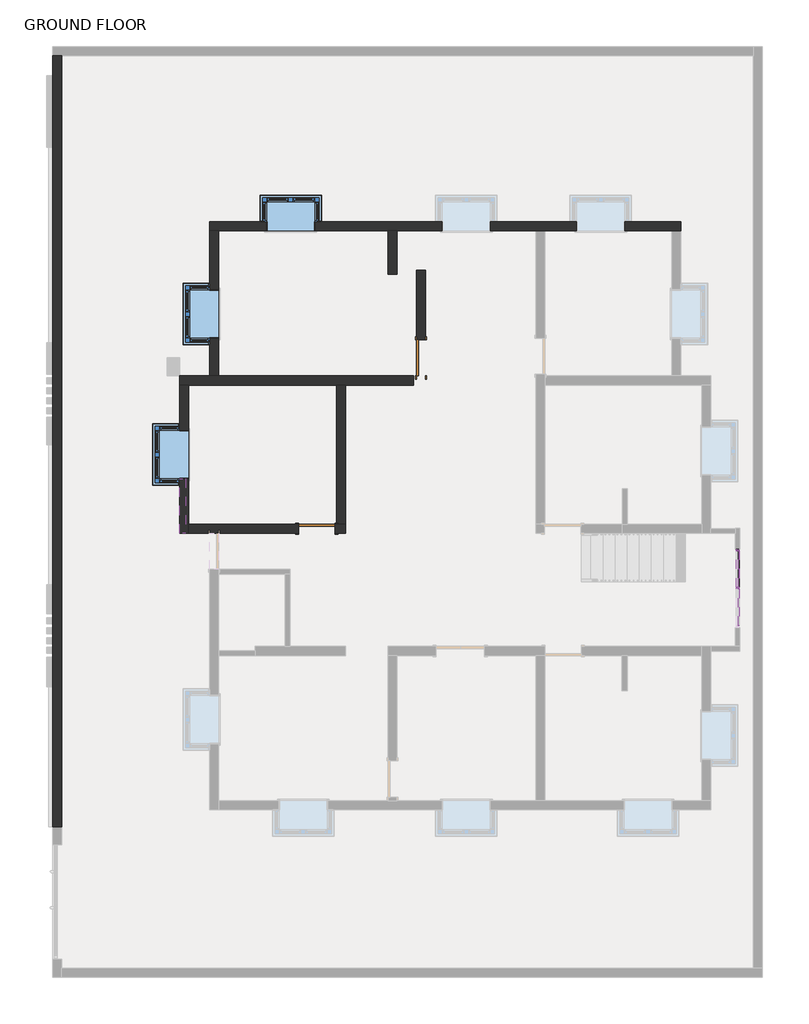
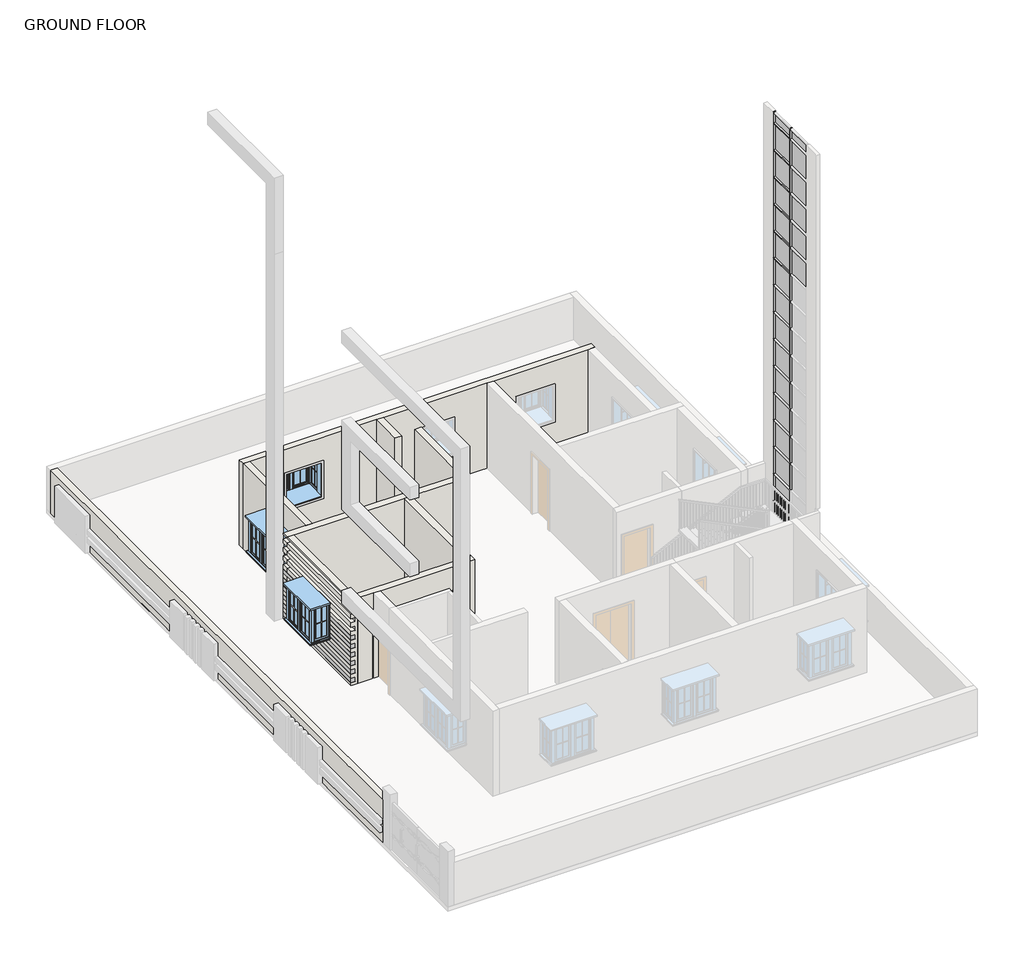
# One storey, part 2 of 5: 38 members, 23 plates, 9 walls, 6 proxies, 3 windows, 2 doors.
"""IFC4 building model written with IfcOpenShell, lengths in millimetres."""

from ifc_helpers import new_model, si_unit, frame, origin, origin_with_axes, place, context, project, spatial, polyline, outline, extrude, faceted_brep, transform, mapped, element, save
from components import door_a90ba1ad, door_0ca8825f, member_c65a811d, member_51048147, member_1ede677d, member_eea045b6, member_18929904, member_e7145701, member_32999801, system_panel_glazed_7f04015b, system_panel_glazed_95b6fecb, window_bay_casement_box_90_degree_angle_4_x4_x2_07b705a1

model = new_model("IFC4")

# Units and contexts
model_context = context("Model", 3, world=origin())
ifc_project = project(units=[si_unit("LENGTHUNIT", "METRE", prefix="MILLI")], contexts=[model_context])

# Site, building, storey
site = spatial("IfcSite", under=ifc_project)
building = spatial("IfcBuilding", under=site)
storey = spatial("IfcBuildingStorey", under=building, Name="GROUND FLOOR", Elevation=0.0)

# Proxies
placement = place(None, origin())
element("IfcBuildingElementProxy", 1, Name="Reveal", ObjectType="Reveal", at=placement, inside=storey, context=model_context, shape_type="SweptSolid", body=[
    extrude(outline(polyline([(-7008.3415084, 4183.133346), (-6855.9415084, 4183.133346), (-6855.9415084, 220.733346), (-7008.3415084, 220.733346), (-7008.3415084, 4183.133346)])), frame((0.0, 0.0, 101.6), z_axis=(0.0, 0.0, 1.0), x_axis=(1.0, 0.0, 0.0)), (0.0, 0.0, 1.0), 152.4),
])
element("IfcBuildingElementProxy", 2, Name="Reveal", ObjectType="Reveal", at=placement, inside=storey, context=model_context, shape_type="SweptSolid", body=[
    extrude(outline(polyline([(-7008.3415084, 4183.133346), (-6855.9415084, 4183.133346), (-6855.9415084, 220.733346), (-7008.3415084, 220.733346), (-7008.3415084, 4183.133346)])), frame((0.0, 0.0, 406.4), z_axis=(0.0, 0.0, 1.0), x_axis=(1.0, 0.0, 0.0)), (0.0, 0.0, 1.0), 152.4),
])
element("IfcBuildingElementProxy", 3, Name="Reveal", ObjectType="Reveal", at=placement, inside=storey, context=model_context, shape_type="SweptSolid", body=[
    extrude(outline(polyline([(-7008.3415084, 4183.133346), (-6855.9415084, 4183.133346), (-6855.9415084, 220.733346), (-7008.3415084, 220.733346), (-7008.3415084, 4183.133346)])), frame((0.0, 0.0, 711.2), z_axis=(0.0, 0.0, 1.0), x_axis=(1.0, 0.0, 0.0)), (0.0, 0.0, 1.0), 152.4),
])
element("IfcBuildingElementProxy", 4, Name="Reveal", ObjectType="Reveal", at=placement, inside=storey, context=model_context, shape_type="SweptSolid", body=[
    extrude(outline(polyline([(-7008.3415084, 1592.333346), (-6855.9415084, 1592.333346), (-6855.9415084, 220.733346), (-7008.3415084, 220.733346), (-7008.3415084, 1592.333346)])), frame((0.0, 0.0, 1016.0), z_axis=(0.0, 0.0, 1.0), x_axis=(1.0, 0.0, 0.0)), (0.0, 0.0, 1.0), 152.4),
    extrude(outline(polyline([(-7008.3415084, 4183.133346), (-6855.9415084, 4183.133346), (-6855.9415084, 2811.533346), (-7008.3415084, 2811.533346), (-7008.3415084, 4183.133346)])), frame((0.0, 0.0, 1016.0), z_axis=(0.0, 0.0, 1.0), x_axis=(1.0, 0.0, 0.0)), (0.0, 0.0, 1.0), 152.4),
])
element("IfcBuildingElementProxy", 5, Name="Reveal", ObjectType="Reveal", at=placement, inside=storey, context=model_context, shape_type="SweptSolid", body=[
    extrude(outline(polyline([(-7008.3415084, 1592.333346), (-6855.9415084, 1592.333346), (-6855.9415084, 220.733346), (-7008.3415084, 220.733346), (-7008.3415084, 1592.333346)])), frame((0.0, 0.0, 1320.8), z_axis=(0.0, 0.0, 1.0), x_axis=(1.0, 0.0, 0.0)), (0.0, 0.0, 1.0), 152.4),
    extrude(outline(polyline([(-7008.3415084, 4183.133346), (-6855.9415084, 4183.133346), (-6855.9415084, 2811.533346), (-7008.3415084, 2811.533346), (-7008.3415084, 4183.133346)])), frame((0.0, 0.0, 1320.8), z_axis=(0.0, 0.0, 1.0), x_axis=(1.0, 0.0, 0.0)), (0.0, 0.0, 1.0), 152.4),
])
element("IfcBuildingElementProxy", 6, Name="Reveal", ObjectType="Reveal", at=placement, inside=storey, context=model_context, shape_type="SweptSolid", body=[
    extrude(outline(polyline([(-7008.3415084, 1592.333346), (-6855.9415084, 1592.333346), (-6855.9415084, 220.733346), (-7008.3415084, 220.733346), (-7008.3415084, 1592.333346)])), frame((0.0, 0.0, 1625.6), z_axis=(0.0, 0.0, 1.0), x_axis=(1.0, 0.0, 0.0)), (0.0, 0.0, 1.0), 152.4),
    extrude(outline(polyline([(-7008.3415084, 4183.133346), (-6855.9415084, 4183.133346), (-6855.9415084, 2811.533346), (-7008.3415084, 2811.533346), (-7008.3415084, 4183.133346)])), frame((0.0, 0.0, 1625.6), z_axis=(0.0, 0.0, 1.0), x_axis=(1.0, 0.0, 0.0)), (0.0, 0.0, 1.0), 152.4),
])

# Doors
door_shape = door_a90ba1ad(model_context)
element("IfcDoor", 7, ObjectType="Single-Flush : 36\" x 84\"", at=placement, inside=storey, context=model_context, shape_type="MappedRepresentation", body=[
    mapped(door_shape, transform((-918.5024437, 4640.333346, 0.0), x_axis=(0.0, -1.0, 0.0), y_axis=(1.0, 0.0, 0.0), z_axis=(0.0, 0.0, 1.0))),
])
door_2_shape = door_0ca8825f(model_context)
element("IfcDoor", 8, ObjectType="Single-Flush : 36\" x 84\"", at=placement, inside=storey, context=model_context, shape_type="MappedRepresentation", body=[
    mapped(door_2_shape, transform((-3541.2415084, 335.033346, 0.0), x_axis=(1.0, 0.0, 0.0), y_axis=(0.0, 1.0, 0.0), z_axis=(0.0, 0.0, 1.0))),
])

# Members
member_shape = member_c65a811d(model_context)
element("IfcMember", 9, ObjectType="Rectangular Mullion : 1.5\" x 2.5\" rectangular", at=placement, inside=storey, context=model_context, shape_type="MappedRepresentation", body=[
    mapped(member_shape, transform((7067.5550459, -219.956654, 0.0), x_axis=(0.0, 0.0, -1.0), y_axis=(-1.0, 0.0, 0.0), z_axis=(0.0, 1.0, 0.0))),
])
member_2_shape = member_51048147(model_context)
element("IfcMember", 10, ObjectType="Rectangular Mullion : 1.5\" x 2.5\" rectangular", at=placement, inside=storey, context=model_context, shape_type="MappedRepresentation", body=[
    mapped(member_2_shape, transform((7067.5550459, -1147.0566543, 10636.25), x_axis=(0.0, 0.0, 1.0), y_axis=(-1.0, 0.0, 0.0), z_axis=(0.0, -1.0, 0.0))),
])
element("IfcMember", 11, ObjectType="Rectangular Mullion : 1.5\" x 2.5\" rectangular", at=placement, inside=storey, context=model_context, shape_type="MappedRepresentation", body=[
    mapped(member_2_shape, transform((7067.5550459, -1147.0566543, 11601.45), x_axis=(0.0, 0.0, 1.0), y_axis=(-1.0, 0.0, 0.0), z_axis=(0.0, -1.0, 0.0))),
])
element("IfcMember", 12, ObjectType="Rectangular Mullion : 1.5\" x 2.5\" rectangular", at=placement, inside=storey, context=model_context, shape_type="MappedRepresentation", body=[
    mapped(member_2_shape, transform((7067.5550459, -1147.0566543, 12566.65), x_axis=(0.0, 0.0, 1.0), y_axis=(-1.0, 0.0, 0.0), z_axis=(0.0, -1.0, 0.0))),
])
element("IfcMember", 13, ObjectType="Rectangular Mullion : 1.5\" x 2.5\" rectangular", at=placement, inside=storey, context=model_context, shape_type="MappedRepresentation", body=[
    mapped(member_2_shape, transform((7067.5550459, -1147.0566543, 13531.85), x_axis=(0.0, 0.0, 1.0), y_axis=(-1.0, 0.0, 0.0), z_axis=(0.0, -1.0, 0.0))),
])
element("IfcMember", 14, ObjectType="Rectangular Mullion : 1.5\" x 2.5\" rectangular", at=placement, inside=storey, context=model_context, shape_type="MappedRepresentation", body=[
    mapped(member_2_shape, transform((7067.5550459, -1147.0566543, 14497.05), x_axis=(0.0, 0.0, 1.0), y_axis=(-1.0, 0.0, 0.0), z_axis=(0.0, -1.0, 0.0))),
])
element("IfcMember", 15, ObjectType="Rectangular Mullion : 1.5\" x 2.5\" rectangular", at=placement, inside=storey, context=model_context, shape_type="MappedRepresentation", body=[
    mapped(member_2_shape, transform((7067.5550459, -1147.0566543, 15462.25), x_axis=(0.0, 0.0, 1.0), y_axis=(-1.0, 0.0, 0.0), z_axis=(0.0, -1.0, 0.0))),
])
member_3_shape = member_1ede677d(model_context)
element("IfcMember", 16, ObjectType="Rectangular Mullion : 1.5\" x 2.5\" rectangular", at=placement, inside=storey, context=model_context, shape_type="MappedRepresentation", body=[
    mapped(member_3_shape, transform((7067.5550459, -1166.1066543, 2914.65), x_axis=(0.0, -1.0, 0.0), y_axis=(-1.0, 0.0, 0.0), z_axis=(0.0, 0.0, -1.0))),
])
element("IfcMember", 17, ObjectType="Rectangular Mullion : 1.5\" x 2.5\" rectangular", at=placement, inside=storey, context=model_context, shape_type="MappedRepresentation", body=[
    mapped(member_3_shape, transform((7067.5550459, -1166.1066543, 3879.85), x_axis=(0.0, -1.0, 0.0), y_axis=(-1.0, 0.0, 0.0), z_axis=(0.0, 0.0, -1.0))),
])
element("IfcMember", 18, ObjectType="Rectangular Mullion : 1.5\" x 2.5\" rectangular", at=placement, inside=storey, context=model_context, shape_type="MappedRepresentation", body=[
    mapped(member_3_shape, transform((7067.5550459, -1166.1066543, 4845.05), x_axis=(0.0, -1.0, 0.0), y_axis=(-1.0, 0.0, 0.0), z_axis=(0.0, 0.0, -1.0))),
])
element("IfcMember", 19, ObjectType="Rectangular Mullion : 1.5\" x 2.5\" rectangular", at=placement, inside=storey, context=model_context, shape_type="MappedRepresentation", body=[
    mapped(member_3_shape, transform((7067.5550459, -1166.1066543, 5810.25), x_axis=(0.0, -1.0, 0.0), y_axis=(-1.0, 0.0, 0.0), z_axis=(0.0, 0.0, -1.0))),
])
element("IfcMember", 20, ObjectType="Rectangular Mullion : 1.5\" x 2.5\" rectangular", at=placement, inside=storey, context=model_context, shape_type="MappedRepresentation", body=[
    mapped(member_3_shape, transform((7067.5550459, -1166.1066543, 6775.45), x_axis=(0.0, -1.0, 0.0), y_axis=(-1.0, 0.0, 0.0), z_axis=(0.0, 0.0, -1.0))),
])
element("IfcMember", 21, ObjectType="Rectangular Mullion : 1.5\" x 2.5\" rectangular", at=placement, inside=storey, context=model_context, shape_type="MappedRepresentation", body=[
    mapped(member_3_shape, transform((7067.5550459, -1166.1066543, 7740.65), x_axis=(0.0, -1.0, 0.0), y_axis=(-1.0, 0.0, 0.0), z_axis=(0.0, 0.0, -1.0))),
])
element("IfcMember", 22, ObjectType="Rectangular Mullion : 1.5\" x 2.5\" rectangular", at=placement, inside=storey, context=model_context, shape_type="MappedRepresentation", body=[
    mapped(member_3_shape, transform((7067.5550459, -1166.1066543, 8705.85), x_axis=(0.0, -1.0, 0.0), y_axis=(-1.0, 0.0, 0.0), z_axis=(0.0, 0.0, -1.0))),
])
element("IfcMember", 23, ObjectType="Rectangular Mullion : 1.5\" x 2.5\" rectangular", at=placement, inside=storey, context=model_context, shape_type="MappedRepresentation", body=[
    mapped(member_3_shape, transform((7067.5550459, -1166.1066543, 9671.05), x_axis=(0.0, -1.0, 0.0), y_axis=(-1.0, 0.0, 0.0), z_axis=(0.0, 0.0, -1.0))),
])
element("IfcMember", 24, ObjectType="Rectangular Mullion : 1.5\" x 2.5\" rectangular", at=placement, inside=storey, context=model_context, shape_type="MappedRepresentation", body=[
    mapped(member_3_shape, transform((7067.5550459, -1166.1066543, 10636.25), x_axis=(0.0, -1.0, 0.0), y_axis=(-1.0, 0.0, 0.0), z_axis=(0.0, 0.0, -1.0))),
])
element("IfcMember", 25, ObjectType="Rectangular Mullion : 1.5\" x 2.5\" rectangular", at=placement, inside=storey, context=model_context, shape_type="MappedRepresentation", body=[
    mapped(member_3_shape, transform((7067.5550459, -1166.1066543, 11601.45), x_axis=(0.0, -1.0, 0.0), y_axis=(-1.0, 0.0, 0.0), z_axis=(0.0, 0.0, -1.0))),
])
element("IfcMember", 26, ObjectType="Rectangular Mullion : 1.5\" x 2.5\" rectangular", at=placement, inside=storey, context=model_context, shape_type="MappedRepresentation", body=[
    mapped(member_3_shape, transform((7067.5550459, -1166.1066543, 12566.65), x_axis=(0.0, -1.0, 0.0), y_axis=(-1.0, 0.0, 0.0), z_axis=(0.0, 0.0, -1.0))),
])
element("IfcMember", 27, ObjectType="Rectangular Mullion : 1.5\" x 2.5\" rectangular", at=placement, inside=storey, context=model_context, shape_type="MappedRepresentation", body=[
    mapped(member_3_shape, transform((7067.5550459, -1166.1066543, 13531.85), x_axis=(0.0, -1.0, 0.0), y_axis=(-1.0, 0.0, 0.0), z_axis=(0.0, 0.0, -1.0))),
])
element("IfcMember", 28, ObjectType="Rectangular Mullion : 1.5\" x 2.5\" rectangular", at=placement, inside=storey, context=model_context, shape_type="MappedRepresentation", body=[
    mapped(member_3_shape, transform((7067.5550459, -1166.1066543, 14497.05), x_axis=(0.0, -1.0, 0.0), y_axis=(-1.0, 0.0, 0.0), z_axis=(0.0, 0.0, -1.0))),
])
member_4_shape = member_eea045b6(model_context)
element("IfcMember", 29, ObjectType="Rectangular Mullion : 1.5\" x 2.5\" rectangular", at=placement, inside=storey, context=model_context, shape_type="MappedRepresentation", body=[
    mapped(member_4_shape, transform((7067.5550459, -1166.1066543, 15462.25), x_axis=(0.0, -1.0, 0.0), y_axis=(-1.0, 0.0, 0.0), z_axis=(0.0, 0.0, -1.0))),
])
member_5_shape = member_18929904(model_context)
element("IfcMember", 30, ObjectType="Rectangular Mullion : 1.5\" x 2.5\" rectangular", at=placement, inside=storey, context=model_context, shape_type="MappedRepresentation", body=[
    mapped(member_5_shape, transform((7067.5550459, -181.856654, 15849.6), x_axis=(0.0, 1.0, 0.0), y_axis=(-1.0, 0.0, 0.0), z_axis=(0.0, 0.0, 1.0))),
])
member_6_shape = member_e7145701(model_context)
element("IfcMember", 31, ObjectType="Rectangular Mullion : 1.5\" x 2.5\" rectangular", at=placement, inside=storey, context=model_context, shape_type="MappedRepresentation", body=[
    mapped(member_6_shape, transform((7067.5550459, -181.856654, 984.25), x_axis=(0.0, 1.0, 0.0), y_axis=(-1.0, 0.0, 0.0), z_axis=(0.0, 0.0, 1.0))),
])
member_7_shape = member_32999801(model_context)
element("IfcMember", 32, ObjectType="Rectangular Mullion : 1.5\" x 2.5\" rectangular", at=placement, inside=storey, context=model_context, shape_type="MappedRepresentation", body=[
    mapped(member_7_shape, transform((7067.5550459, -181.856654, 1949.45), x_axis=(0.0, 1.0, 0.0), y_axis=(-1.0, 0.0, 0.0), z_axis=(0.0, 0.0, 1.0))),
])
element("IfcMember", 33, ObjectType="Rectangular Mullion : 1.5\" x 2.5\" rectangular", at=placement, inside=storey, context=model_context, shape_type="MappedRepresentation", body=[
    mapped(member_7_shape, transform((7067.5550459, -181.856654, 2914.65), x_axis=(0.0, 1.0, 0.0), y_axis=(-1.0, 0.0, 0.0), z_axis=(0.0, 0.0, 1.0))),
])
element("IfcMember", 34, ObjectType="Rectangular Mullion : 1.5\" x 2.5\" rectangular", at=placement, inside=storey, context=model_context, shape_type="MappedRepresentation", body=[
    mapped(member_7_shape, transform((7067.5550459, -181.856654, 3879.85), x_axis=(0.0, 1.0, 0.0), y_axis=(-1.0, 0.0, 0.0), z_axis=(0.0, 0.0, 1.0))),
])
element("IfcMember", 35, ObjectType="Rectangular Mullion : 1.5\" x 2.5\" rectangular", at=placement, inside=storey, context=model_context, shape_type="MappedRepresentation", body=[
    mapped(member_7_shape, transform((7067.5550459, -181.856654, 4845.05), x_axis=(0.0, 1.0, 0.0), y_axis=(-1.0, 0.0, 0.0), z_axis=(0.0, 0.0, 1.0))),
])
element("IfcMember", 36, ObjectType="Rectangular Mullion : 1.5\" x 2.5\" rectangular", at=placement, inside=storey, context=model_context, shape_type="MappedRepresentation", body=[
    mapped(member_7_shape, transform((7067.5550459, -181.856654, 5810.25), x_axis=(0.0, 1.0, 0.0), y_axis=(-1.0, 0.0, 0.0), z_axis=(0.0, 0.0, 1.0))),
])
element("IfcMember", 37, ObjectType="Rectangular Mullion : 1.5\" x 2.5\" rectangular", at=placement, inside=storey, context=model_context, shape_type="MappedRepresentation", body=[
    mapped(member_7_shape, transform((7067.5550459, -181.856654, 6775.45), x_axis=(0.0, 1.0, 0.0), y_axis=(-1.0, 0.0, 0.0), z_axis=(0.0, 0.0, 1.0))),
])
element("IfcMember", 38, ObjectType="Rectangular Mullion : 1.5\" x 2.5\" rectangular", at=placement, inside=storey, context=model_context, shape_type="MappedRepresentation", body=[
    mapped(member_7_shape, transform((7067.5550459, -181.856654, 7740.65), x_axis=(0.0, 1.0, 0.0), y_axis=(-1.0, 0.0, 0.0), z_axis=(0.0, 0.0, 1.0))),
])
element("IfcMember", 39, ObjectType="Rectangular Mullion : 1.5\" x 2.5\" rectangular", at=placement, inside=storey, context=model_context, shape_type="MappedRepresentation", body=[
    mapped(member_7_shape, transform((7067.5550459, -181.856654, 8705.85), x_axis=(0.0, 1.0, 0.0), y_axis=(-1.0, 0.0, 0.0), z_axis=(0.0, 0.0, 1.0))),
])
element("IfcMember", 40, ObjectType="Rectangular Mullion : 1.5\" x 2.5\" rectangular", at=placement, inside=storey, context=model_context, shape_type="MappedRepresentation", body=[
    mapped(member_7_shape, transform((7067.5550459, -181.856654, 9671.05), x_axis=(0.0, 1.0, 0.0), y_axis=(-1.0, 0.0, 0.0), z_axis=(0.0, 0.0, 1.0))),
])
element("IfcMember", 41, ObjectType="Rectangular Mullion : 1.5\" x 2.5\" rectangular", at=placement, inside=storey, context=model_context, shape_type="MappedRepresentation", body=[
    mapped(member_7_shape, transform((7067.5550459, -181.856654, 10636.25), x_axis=(0.0, 1.0, 0.0), y_axis=(-1.0, 0.0, 0.0), z_axis=(0.0, 0.0, 1.0))),
])
element("IfcMember", 42, ObjectType="Rectangular Mullion : 1.5\" x 2.5\" rectangular", at=placement, inside=storey, context=model_context, shape_type="MappedRepresentation", body=[
    mapped(member_7_shape, transform((7067.5550459, -181.856654, 11601.45), x_axis=(0.0, 1.0, 0.0), y_axis=(-1.0, 0.0, 0.0), z_axis=(0.0, 0.0, 1.0))),
])
element("IfcMember", 43, ObjectType="Rectangular Mullion : 1.5\" x 2.5\" rectangular", at=placement, inside=storey, context=model_context, shape_type="MappedRepresentation", body=[
    mapped(member_7_shape, transform((7067.5550459, -181.856654, 12566.65), x_axis=(0.0, 1.0, 0.0), y_axis=(-1.0, 0.0, 0.0), z_axis=(0.0, 0.0, 1.0))),
])
element("IfcMember", 44, ObjectType="Rectangular Mullion : 1.5\" x 2.5\" rectangular", at=placement, inside=storey, context=model_context, shape_type="MappedRepresentation", body=[
    mapped(member_7_shape, transform((7067.5550459, -181.856654, 13531.85), x_axis=(0.0, 1.0, 0.0), y_axis=(-1.0, 0.0, 0.0), z_axis=(0.0, 0.0, 1.0))),
])
element("IfcMember", 45, ObjectType="Rectangular Mullion : 1.5\" x 2.5\" rectangular", at=placement, inside=storey, context=model_context, shape_type="MappedRepresentation", body=[
    mapped(member_7_shape, transform((7067.5550459, -181.856654, 14497.05), x_axis=(0.0, 1.0, 0.0), y_axis=(-1.0, 0.0, 0.0), z_axis=(0.0, 0.0, 1.0))),
])
element("IfcMember", 46, ObjectType="Rectangular Mullion : 1.5\" x 2.5\" rectangular", at=placement, inside=storey, context=model_context, shape_type="MappedRepresentation", body=[
    mapped(member_7_shape, transform((7067.5550459, -181.856654, 15462.25), x_axis=(0.0, 1.0, 0.0), y_axis=(-1.0, 0.0, 0.0), z_axis=(0.0, 0.0, 1.0))),
])

# Plates
system_panel_glazed_shape = system_panel_glazed_7f04015b(model_context)
element("IfcPlate", 47, ObjectType="System Panel : Glazed", at=placement, inside=storey, context=model_context, shape_type="MappedRepresentation", body=[
    mapped(system_panel_glazed_shape, transform((7067.5550459, -683.5066541, 38.1), x_axis=(0.0, -1.0, 0.0), y_axis=(1.0, 0.0, 0.0), z_axis=(0.0, 0.0, 1.0))),
])
element("IfcPlate", 48, ObjectType="System Panel : Glazed", at=placement, inside=storey, context=model_context, shape_type="MappedRepresentation", body=[
    mapped(system_panel_glazed_shape, transform((7067.5550459, -683.5066541, 1003.3), x_axis=(0.0, -1.0, 0.0), y_axis=(1.0, 0.0, 0.0), z_axis=(0.0, 0.0, 1.0))),
])
element("IfcPlate", 49, ObjectType="System Panel : Glazed", at=placement, inside=storey, context=model_context, shape_type="MappedRepresentation", body=[
    mapped(system_panel_glazed_shape, transform((7067.5550459, -683.5066541, 1968.5), x_axis=(0.0, -1.0, 0.0), y_axis=(1.0, 0.0, 0.0), z_axis=(0.0, 0.0, 1.0))),
])
element("IfcPlate", 50, ObjectType="System Panel : Glazed", at=placement, inside=storey, context=model_context, shape_type="MappedRepresentation", body=[
    mapped(system_panel_glazed_shape, transform((7067.5550459, -683.5066541, 2933.7), x_axis=(0.0, -1.0, 0.0), y_axis=(1.0, 0.0, 0.0), z_axis=(0.0, 0.0, 1.0))),
])
element("IfcPlate", 51, ObjectType="System Panel : Glazed", at=placement, inside=storey, context=model_context, shape_type="MappedRepresentation", body=[
    mapped(system_panel_glazed_shape, transform((7067.5550459, -683.5066541, 3898.9), x_axis=(0.0, -1.0, 0.0), y_axis=(1.0, 0.0, 0.0), z_axis=(0.0, 0.0, 1.0))),
])
element("IfcPlate", 52, ObjectType="System Panel : Glazed", at=placement, inside=storey, context=model_context, shape_type="MappedRepresentation", body=[
    mapped(system_panel_glazed_shape, transform((7067.5550459, -683.5066541, 4864.1), x_axis=(0.0, -1.0, 0.0), y_axis=(1.0, 0.0, 0.0), z_axis=(0.0, 0.0, 1.0))),
])
element("IfcPlate", 53, ObjectType="System Panel : Glazed", at=placement, inside=storey, context=model_context, shape_type="MappedRepresentation", body=[
    mapped(system_panel_glazed_shape, transform((7067.5550459, -683.5066541, 5829.3), x_axis=(0.0, -1.0, 0.0), y_axis=(1.0, 0.0, 0.0), z_axis=(0.0, 0.0, 1.0))),
])
element("IfcPlate", 54, ObjectType="System Panel : Glazed", at=placement, inside=storey, context=model_context, shape_type="MappedRepresentation", body=[
    mapped(system_panel_glazed_shape, transform((7067.5550459, -683.5066541, 6794.5), x_axis=(0.0, -1.0, 0.0), y_axis=(1.0, 0.0, 0.0), z_axis=(0.0, 0.0, 1.0))),
])
element("IfcPlate", 55, ObjectType="System Panel : Glazed", at=placement, inside=storey, context=model_context, shape_type="MappedRepresentation", body=[
    mapped(system_panel_glazed_shape, transform((7067.5550459, -683.5066541, 7759.7), x_axis=(0.0, -1.0, 0.0), y_axis=(1.0, 0.0, 0.0), z_axis=(0.0, 0.0, 1.0))),
])
element("IfcPlate", 56, ObjectType="System Panel : Glazed", at=placement, inside=storey, context=model_context, shape_type="MappedRepresentation", body=[
    mapped(system_panel_glazed_shape, transform((7067.5550459, -683.5066541, 8724.9), x_axis=(0.0, -1.0, 0.0), y_axis=(1.0, 0.0, 0.0), z_axis=(0.0, 0.0, 1.0))),
])
element("IfcPlate", 57, ObjectType="System Panel : Glazed", at=placement, inside=storey, context=model_context, shape_type="MappedRepresentation", body=[
    mapped(system_panel_glazed_shape, transform((7067.5550459, -683.5066541, 9690.1), x_axis=(0.0, -1.0, 0.0), y_axis=(1.0, 0.0, 0.0), z_axis=(0.0, 0.0, 1.0))),
])
element("IfcPlate", 58, ObjectType="System Panel : Glazed", at=placement, inside=storey, context=model_context, shape_type="MappedRepresentation", body=[
    mapped(system_panel_glazed_shape, transform((7067.5550459, -683.5066541, 10655.3), x_axis=(0.0, -1.0, 0.0), y_axis=(1.0, 0.0, 0.0), z_axis=(0.0, 0.0, 1.0))),
])
element("IfcPlate", 59, ObjectType="System Panel : Glazed", at=placement, inside=storey, context=model_context, shape_type="MappedRepresentation", body=[
    mapped(system_panel_glazed_shape, transform((7067.5550459, -1648.7066543, 10655.3), x_axis=(0.0, -1.0, 0.0), y_axis=(1.0, 0.0, 0.0), z_axis=(0.0, 0.0, 1.0))),
])
element("IfcPlate", 60, ObjectType="System Panel : Glazed", at=placement, inside=storey, context=model_context, shape_type="MappedRepresentation", body=[
    mapped(system_panel_glazed_shape, transform((7067.5550459, -683.5066541, 11620.5), x_axis=(0.0, -1.0, 0.0), y_axis=(1.0, 0.0, 0.0), z_axis=(0.0, 0.0, 1.0))),
])
element("IfcPlate", 61, ObjectType="System Panel : Glazed", at=placement, inside=storey, context=model_context, shape_type="MappedRepresentation", body=[
    mapped(system_panel_glazed_shape, transform((7067.5550459, -1648.7066543, 11620.5), x_axis=(0.0, -1.0, 0.0), y_axis=(1.0, 0.0, 0.0), z_axis=(0.0, 0.0, 1.0))),
])
element("IfcPlate", 62, ObjectType="System Panel : Glazed", at=placement, inside=storey, context=model_context, shape_type="MappedRepresentation", body=[
    mapped(system_panel_glazed_shape, transform((7067.5550459, -683.5066541, 12585.7), x_axis=(0.0, -1.0, 0.0), y_axis=(1.0, 0.0, 0.0), z_axis=(0.0, 0.0, 1.0))),
])
element("IfcPlate", 63, ObjectType="System Panel : Glazed", at=placement, inside=storey, context=model_context, shape_type="MappedRepresentation", body=[
    mapped(system_panel_glazed_shape, transform((7067.5550459, -1648.7066543, 12585.7), x_axis=(0.0, -1.0, 0.0), y_axis=(1.0, 0.0, 0.0), z_axis=(0.0, 0.0, 1.0))),
])
element("IfcPlate", 64, ObjectType="System Panel : Glazed", at=placement, inside=storey, context=model_context, shape_type="MappedRepresentation", body=[
    mapped(system_panel_glazed_shape, transform((7067.5550459, -683.5066541, 13550.9), x_axis=(0.0, -1.0, 0.0), y_axis=(1.0, 0.0, 0.0), z_axis=(0.0, 0.0, 1.0))),
])
element("IfcPlate", 65, ObjectType="System Panel : Glazed", at=placement, inside=storey, context=model_context, shape_type="MappedRepresentation", body=[
    mapped(system_panel_glazed_shape, transform((7067.5550459, -1648.7066543, 13550.9), x_axis=(0.0, -1.0, 0.0), y_axis=(1.0, 0.0, 0.0), z_axis=(0.0, 0.0, 1.0))),
])
element("IfcPlate", 66, ObjectType="System Panel : Glazed", at=placement, inside=storey, context=model_context, shape_type="MappedRepresentation", body=[
    mapped(system_panel_glazed_shape, transform((7067.5550459, -683.5066541, 14516.1), x_axis=(0.0, -1.0, 0.0), y_axis=(1.0, 0.0, 0.0), z_axis=(0.0, 0.0, 1.0))),
])
element("IfcPlate", 67, ObjectType="System Panel : Glazed", at=placement, inside=storey, context=model_context, shape_type="MappedRepresentation", body=[
    mapped(system_panel_glazed_shape, transform((7067.5550459, -1648.7066543, 14516.1), x_axis=(0.0, -1.0, 0.0), y_axis=(1.0, 0.0, 0.0), z_axis=(0.0, 0.0, 1.0))),
])
system_panel_glazed_2_shape = system_panel_glazed_95b6fecb(model_context)
element("IfcPlate", 68, ObjectType="System Panel : Glazed", at=placement, inside=storey, context=model_context, shape_type="MappedRepresentation", body=[
    mapped(system_panel_glazed_2_shape, transform((7067.5550459, -683.5066541, 15481.3), x_axis=(0.0, -1.0, 0.0), y_axis=(1.0, 0.0, 0.0), z_axis=(0.0, 0.0, 1.0))),
])
element("IfcPlate", 69, ObjectType="System Panel : Glazed", at=placement, inside=storey, context=model_context, shape_type="MappedRepresentation", body=[
    mapped(system_panel_glazed_2_shape, transform((7067.5550459, -1648.7066543, 15481.3), x_axis=(0.0, -1.0, 0.0), y_axis=(1.0, 0.0, 0.0), z_axis=(0.0, 0.0, 1.0))),
])

# Walls
element("IfcWall", 70, ObjectType="9\"", at=placement, inside=storey, context=model_context, shape_type="Brep", body=[
    faceted_brep([(5640.8584916, 8069.333346, 0.0), (-6246.3415084, 8069.333346, 0.0), (-6246.3415084, 8069.333346, 3048.0), (5640.8584916, 8069.333346, 3048.0), (-3592.0415084, 8069.333346, 2184.4), (-4811.2415084, 8069.333346, 2184.4), (-4811.2415084, 8069.333346, 914.4), (-3592.0415084, 8069.333346, 914.4), (4231.1584916, 8069.333346, 2184.4), (3011.9584916, 8069.333346, 2184.4), (3011.9584916, 8069.333346, 914.4), (4231.1584916, 8069.333346, 914.4), (840.2584916, 8069.333346, 2184.4), (-378.9415084, 8069.333346, 2184.4), (-378.9415084, 8069.333346, 914.4), (840.2584916, 8069.333346, 914.4), (5640.8584916, 7840.733346, 0.0), (5640.8584916, 7840.733346, 3048.0), (5412.2584916, 7840.733346, 3048.0), (2211.8584916, 7840.733346, 3048.0), (1983.2584916, 7840.733346, 3048.0), (-1521.9415084, 7840.733346, 3048.0), (-1750.5415084, 7840.733346, 3048.0), (-6017.7415084, 7840.733346, 3048.0), (-6246.3415084, 7840.733346, 3048.0), (-6246.3415084, 7840.733346, 0.0), (-6017.7415084, 7840.733346, 0.0), (-1750.5415084, 7840.733346, 0.0), (-1521.9415084, 7840.733346, 0.0), (1983.2584916, 7840.733346, 0.0), (2211.8584916, 7840.733346, 0.0), (5412.2584916, 7840.733346, 0.0), (-3592.0415084, 7840.733346, 2184.4), (-3592.0415084, 7840.733346, 914.4), (-4811.2415084, 7840.733346, 914.4), (-4811.2415084, 7840.733346, 2184.4), (4231.1584916, 7840.733346, 2184.4), (4231.1584916, 7840.733346, 914.4), (3011.9584916, 7840.733346, 914.4), (3011.9584916, 7840.733346, 2184.4), (840.2584916, 7840.733346, 2184.4), (840.2584916, 7840.733346, 914.4), (-378.9415084, 7840.733346, 914.4), (-378.9415084, 7840.733346, 2184.4)], [[[0, 1, 2, 3], [4, 5, 6, 7], [8, 9, 10, 11], [12, 13, 14, 15]], [[16, 17, 18, 19, 20, 21, 22, 23, 24, 25, 26, 27, 28, 29, 30, 31], [32, 33, 34, 35], [36, 37, 38, 39], [40, 41, 42, 43]], [[1, 0, 16, 31, 30, 29, 28, 27, 26, 25]], [[3, 2, 24, 23, 22, 21, 20, 19, 18, 17]], [[2, 1, 25, 24]], [[0, 3, 17, 16]], [[33, 32, 4, 7]], [[34, 33, 7, 6]], [[35, 34, 6, 5]], [[32, 35, 5, 4]], [[37, 36, 8, 11]], [[38, 37, 11, 10]], [[39, 38, 10, 9]], [[36, 39, 9, 8]], [[41, 40, 12, 15]], [[42, 41, 15, 14]], [[43, 42, 14, 13]], [[40, 43, 13, 12]]]),
])
element("IfcWall", 71, ObjectType="9\"", at=placement, inside=storey, context=model_context, shape_type="SweptSolid", body=[
    extrude(outline(polyline([(7840.733346, 0.0), (4183.133346, 0.0), (4183.133346, 3048.0), (7840.733346, 3048.0), (7840.733346, 0.0)]), holes=[polyline([(6354.833346, 2184.4), (5135.633346, 2184.4), (5135.633346, 914.4), (6354.833346, 914.4), (6354.833346, 2184.4)])]), frame((-6246.3415084, 0.0, 0.0), z_axis=(1.0, 0.0, 0.0), x_axis=(0.0, 1.0, 0.0)), (0.0, 0.0, 1.0), 228.6),
])
element("IfcWall", 72, ObjectType="9\"", at=placement, inside=storey, context=model_context, shape_type="SweptSolid", body=[
    extrude(outline(polyline([(-1750.5415084, 6747.0175593), (-1750.5415084, 7840.733346), (-1521.9415084, 7840.733346), (-1521.9415084, 6747.0175593), (-1750.5415084, 6747.0175593)])), origin_with_axes(), (0.0, 0.0, 1.0), 3048.0),
])
element("IfcWall", 73, ObjectType="9\"", at=placement, inside=storey, context=model_context, shape_type="Brep", body=[
    faceted_brep([(-1108.4404612, 4183.133346, 0.0), (-6017.7415084, 4183.133346, 0.0), (-6246.3415084, 4183.133346, 0.0), (-7008.3415084, 4183.133346, 0.0), (-7008.3415084, 4183.133346, 101.6), (-6855.9415084, 4183.133346, 101.6), (-6855.9415084, 4183.133346, 254.0), (-7008.3415084, 4183.133346, 254.0), (-7008.3415084, 4183.133346, 406.4), (-6855.9415084, 4183.133346, 406.4), (-6855.9415084, 4183.133346, 558.8), (-7008.3415084, 4183.133346, 558.8), (-7008.3415084, 4183.133346, 711.2), (-6855.9415084, 4183.133346, 711.2), (-6855.9415084, 4183.133346, 863.6), (-7008.3415084, 4183.133346, 863.6), (-7008.3415084, 4183.133346, 1016.0), (-6855.9415084, 4183.133346, 1016.0), (-6855.9415084, 4183.133346, 1168.4), (-7008.3415084, 4183.133346, 1168.4), (-7008.3415084, 4183.133346, 1320.8), (-6855.9415084, 4183.133346, 1320.8), (-6855.9415084, 4183.133346, 1473.2), (-7008.3415084, 4183.133346, 1473.2), (-7008.3415084, 4183.133346, 1625.6), (-6855.9415084, 4183.133346, 1625.6), (-6855.9415084, 4183.133346, 1778.0), (-7008.3415084, 4183.133346, 1778.0), (-7008.3415084, 4183.133346, 1930.4), (-6855.9415084, 4183.133346, 1930.4), (-6855.9415084, 4183.133346, 2082.8), (-7008.3415084, 4183.133346, 2082.8), (-7008.3415084, 4183.133346, 2235.2), (-6855.9415084, 4183.133346, 2235.2), (-6855.9415084, 4183.133346, 2387.6), (-7008.3415084, 4183.133346, 2387.6), (-7008.3415084, 4183.133346, 2540.0), (-6855.9415084, 4183.133346, 2540.0), (-6855.9415084, 4183.133346, 2692.4), (-7008.3415084, 4183.133346, 2692.4), (-7008.3415084, 4183.133346, 2844.8), (-6855.9415084, 4183.133346, 2844.8), (-6855.9415084, 4183.133346, 2997.2), (-7008.3415084, 4183.133346, 2997.2), (-7008.3415084, 4183.133346, 3048.0), (-6246.3415084, 4183.133346, 3048.0), (-6017.7415084, 4183.133346, 3048.0), (-1108.4404612, 4183.133346, 3048.0), (-7008.3415084, 3954.533346, 0.0), (-6779.7415084, 3954.533346, 0.0), (-3045.9415084, 3954.533346, 0.0), (-2817.3415084, 3954.533346, 0.0), (-1108.4404612, 3954.533346, 0.0), (-1108.4404612, 3954.533346, 3048.0), (-2817.3415084, 3954.533346, 3048.0), (-3045.9415084, 3954.533346, 3048.0), (-6779.7415084, 3954.533346, 3048.0), (-7008.3415084, 3954.533346, 3048.0), (-7008.3415084, 3954.533346, 2997.2), (-6855.9415084, 3954.533346, 2997.2), (-6855.9415084, 3954.533346, 2844.8), (-7008.3415084, 3954.533346, 2844.8), (-7008.3415084, 3954.533346, 2692.4), (-6855.9415084, 3954.533346, 2692.4), (-6855.9415084, 3954.533346, 2540.0), (-7008.3415084, 3954.533346, 2540.0), (-7008.3415084, 3954.533346, 2387.6), (-6855.9415084, 3954.533346, 2387.6), (-6855.9415084, 3954.533346, 2235.2), (-7008.3415084, 3954.533346, 2235.2), (-7008.3415084, 3954.533346, 2082.8), (-6855.9415084, 3954.533346, 2082.8), (-6855.9415084, 3954.533346, 1930.4), (-7008.3415084, 3954.533346, 1930.4), (-7008.3415084, 3954.533346, 1778.0), (-6855.9415084, 3954.533346, 1778.0), (-6855.9415084, 3954.533346, 1625.6), (-7008.3415084, 3954.533346, 1625.6), (-7008.3415084, 3954.533346, 1473.2), (-6855.9415084, 3954.533346, 1473.2), (-6855.9415084, 3954.533346, 1320.8), (-7008.3415084, 3954.533346, 1320.8), (-7008.3415084, 3954.533346, 1168.4), (-6855.9415084, 3954.533346, 1168.4), (-6855.9415084, 3954.533346, 1016.0), (-7008.3415084, 3954.533346, 1016.0), (-7008.3415084, 3954.533346, 863.6), (-6855.9415084, 3954.533346, 863.6), (-6855.9415084, 3954.533346, 711.2), (-7008.3415084, 3954.533346, 711.2), (-7008.3415084, 3954.533346, 558.8), (-6855.9415084, 3954.533346, 558.8), (-6855.9415084, 3954.533346, 406.4), (-7008.3415084, 3954.533346, 406.4), (-7008.3415084, 3954.533346, 254.0), (-6855.9415084, 3954.533346, 254.0), (-6855.9415084, 3954.533346, 101.6), (-7008.3415084, 3954.533346, 101.6)], [[[0, 1, 2, 3, 4, 5, 6, 7, 8, 9, 10, 11, 12, 13, 14, 15, 16, 17, 18, 19, 20, 21, 22, 23, 24, 25, 26, 27, 28, 29, 30, 31, 32, 33, 34, 35, 36, 37, 38, 39, 40, 41, 42, 43, 44, 45, 46, 47]], [[48, 49, 50, 51, 52, 53, 54, 55, 56, 57, 58, 59, 60, 61, 62, 63, 64, 65, 66, 67, 68, 69, 70, 71, 72, 73, 74, 75, 76, 77, 78, 79, 80, 81, 82, 83, 84, 85, 86, 87, 88, 89, 90, 91, 92, 93, 94, 95, 96, 97]], [[3, 2, 1, 0, 52, 51, 50, 49, 48]], [[47, 46, 45, 44, 57, 56, 55, 54, 53]], [[0, 47, 53, 52]], [[3, 48, 97, 4]], [[57, 44, 43, 58]], [[7, 94, 93, 8]], [[11, 90, 89, 12]], [[61, 40, 39, 62]], [[65, 36, 35, 66]], [[69, 32, 31, 70]], [[73, 28, 27, 74]], [[77, 24, 23, 78]], [[81, 20, 19, 82]], [[85, 16, 15, 86]], [[6, 95, 94, 7]], [[95, 6, 5, 96]], [[96, 5, 4, 97]], [[10, 91, 90, 11]], [[91, 10, 9, 92]], [[92, 9, 8, 93]], [[42, 59, 58, 43]], [[59, 42, 41, 60]], [[60, 41, 40, 61]], [[38, 63, 62, 39]], [[63, 38, 37, 64]], [[64, 37, 36, 65]], [[34, 67, 66, 35]], [[67, 34, 33, 68]], [[68, 33, 32, 69]], [[30, 71, 70, 31]], [[71, 30, 29, 72]], [[72, 29, 28, 73]], [[26, 75, 74, 27]], [[75, 26, 25, 76]], [[76, 25, 24, 77]], [[22, 79, 78, 23]], [[79, 22, 21, 80]], [[80, 21, 20, 81]], [[18, 83, 82, 19]], [[83, 18, 17, 84]], [[84, 17, 16, 85]], [[14, 87, 86, 15]], [[87, 14, 13, 88]], [[88, 13, 12, 89]]]),
])
element("IfcWall", 74, ObjectType="9\"", at=placement, inside=storey, context=model_context, shape_type="Brep", body=[
    faceted_brep([(-7008.3415084, 3954.533346, 0.0), (-7008.3415084, 220.733346, 0.0), (-7008.3415084, 220.733346, 101.6), (-7008.3415084, 3954.533346, 101.6), (-7008.3415084, 220.733346, 3048.0), (-7008.3415084, 3954.533346, 3048.0), (-7008.3415084, 3954.533346, 2997.2), (-7008.3415084, 220.733346, 2997.2), (-7008.3415084, 1592.333346, 914.4), (-7008.3415084, 2811.533346, 914.4), (-7008.3415084, 2811.533346, 1016.0), (-7008.3415084, 3954.533346, 1016.0), (-7008.3415084, 3954.533346, 863.6), (-7008.3415084, 220.733346, 863.6), (-7008.3415084, 220.733346, 1016.0), (-7008.3415084, 1592.333346, 1016.0), (-7008.3415084, 2811.533346, 2184.4), (-7008.3415084, 1592.333346, 2184.4), (-7008.3415084, 1592.333346, 2082.8), (-7008.3415084, 220.733346, 2082.8), (-7008.3415084, 220.733346, 2235.2), (-7008.3415084, 3954.533346, 2235.2), (-7008.3415084, 3954.533346, 2082.8), (-7008.3415084, 2811.533346, 2082.8), (-7008.3415084, 3954.533346, 254.0), (-7008.3415084, 220.733346, 254.0), (-7008.3415084, 220.733346, 406.4), (-7008.3415084, 3954.533346, 406.4), (-7008.3415084, 3954.533346, 558.8), (-7008.3415084, 220.733346, 558.8), (-7008.3415084, 220.733346, 711.2), (-7008.3415084, 3954.533346, 711.2), (-7008.3415084, 220.733346, 2844.8), (-7008.3415084, 3954.533346, 2844.8), (-7008.3415084, 3954.533346, 2692.4), (-7008.3415084, 220.733346, 2692.4), (-7008.3415084, 220.733346, 2540.0), (-7008.3415084, 3954.533346, 2540.0), (-7008.3415084, 3954.533346, 2387.6), (-7008.3415084, 220.733346, 2387.6), (-7008.3415084, 220.733346, 1930.4), (-7008.3415084, 1592.333346, 1930.4), (-7008.3415084, 1592.333346, 1778.0), (-7008.3415084, 220.733346, 1778.0), (-7008.3415084, 2811.533346, 1930.4), (-7008.3415084, 3954.533346, 1930.4), (-7008.3415084, 3954.533346, 1778.0), (-7008.3415084, 2811.533346, 1778.0), (-7008.3415084, 220.733346, 1625.6), (-7008.3415084, 1592.333346, 1625.6), (-7008.3415084, 1592.333346, 1473.2), (-7008.3415084, 220.733346, 1473.2), (-7008.3415084, 2811.533346, 1625.6), (-7008.3415084, 3954.533346, 1625.6), (-7008.3415084, 3954.533346, 1473.2), (-7008.3415084, 2811.533346, 1473.2), (-7008.3415084, 220.733346, 1320.8), (-7008.3415084, 1592.333346, 1320.8), (-7008.3415084, 1592.333346, 1168.4), (-7008.3415084, 220.733346, 1168.4), (-7008.3415084, 2811.533346, 1320.8), (-7008.3415084, 3954.533346, 1320.8), (-7008.3415084, 3954.533346, 1168.4), (-7008.3415084, 2811.533346, 1168.4), (-6779.7415084, 220.733346, 0.0), (-6779.7415084, 449.333346, 0.0), (-6779.7415084, 3954.533346, 0.0), (-6779.7415084, 3954.533346, 3048.0), (-6779.7415084, 449.333346, 3048.0), (-6779.7415084, 220.733346, 3048.0), (-6779.7415084, 2811.533346, 2184.4), (-6779.7415084, 2811.533346, 914.4), (-6779.7415084, 1592.333346, 914.4), (-6779.7415084, 1592.333346, 2184.4), (-6855.9415084, 3954.533346, 101.6), (-6855.9415084, 3954.533346, 254.0), (-6855.9415084, 3954.533346, 406.4), (-6855.9415084, 3954.533346, 558.8), (-6855.9415084, 3954.533346, 711.2), (-6855.9415084, 3954.533346, 863.6), (-6855.9415084, 3954.533346, 1016.0), (-6855.9415084, 3954.533346, 1168.4), (-6855.9415084, 3954.533346, 1320.8), (-6855.9415084, 3954.533346, 1473.2), (-6855.9415084, 3954.533346, 1625.6), (-6855.9415084, 3954.533346, 1778.0), (-6855.9415084, 3954.533346, 1930.4), (-6855.9415084, 3954.533346, 2082.8), (-6855.9415084, 3954.533346, 2235.2), (-6855.9415084, 3954.533346, 2387.6), (-6855.9415084, 3954.533346, 2540.0), (-6855.9415084, 3954.533346, 2692.4), (-6855.9415084, 3954.533346, 2844.8), (-6855.9415084, 3954.533346, 2997.2), (-6855.9415084, 220.733346, 2997.2), (-6855.9415084, 220.733346, 2844.8), (-6855.9415084, 220.733346, 2692.4), (-6855.9415084, 220.733346, 2540.0), (-6855.9415084, 220.733346, 2387.6), (-6855.9415084, 220.733346, 2235.2), (-6855.9415084, 220.733346, 2082.8), (-6855.9415084, 220.733346, 1930.4), (-6855.9415084, 220.733346, 1778.0), (-6855.9415084, 220.733346, 1625.6), (-6855.9415084, 220.733346, 1473.2), (-6855.9415084, 220.733346, 1320.8), (-6855.9415084, 220.733346, 1168.4), (-6855.9415084, 220.733346, 1016.0), (-6855.9415084, 220.733346, 863.6), (-6855.9415084, 220.733346, 711.2), (-6855.9415084, 220.733346, 558.8), (-6855.9415084, 220.733346, 406.4), (-6855.9415084, 220.733346, 254.0), (-6855.9415084, 220.733346, 101.6), (-6855.9415084, 2811.533346, 2082.8), (-6855.9415084, 2811.533346, 1930.4), (-6855.9415084, 2811.533346, 1778.0), (-6855.9415084, 2811.533346, 1625.6), (-6855.9415084, 2811.533346, 1473.2), (-6855.9415084, 2811.533346, 1320.8), (-6855.9415084, 2811.533346, 1168.4), (-6855.9415084, 2811.533346, 1016.0), (-6855.9415084, 1592.333346, 1016.0), (-6855.9415084, 1592.333346, 1168.4), (-6855.9415084, 1592.333346, 1320.8), (-6855.9415084, 1592.333346, 1473.2), (-6855.9415084, 1592.333346, 1625.6), (-6855.9415084, 1592.333346, 1778.0), (-6855.9415084, 1592.333346, 1930.4), (-6855.9415084, 1592.333346, 2082.8)], [[[0, 1, 2, 3]], [[4, 5, 6, 7]], [[8, 9, 10, 11, 12, 13, 14, 15]], [[16, 17, 18, 19, 20, 21, 22, 23]], [[24, 25, 26, 27]], [[28, 29, 30, 31]], [[32, 33, 34, 35]], [[36, 37, 38, 39]], [[40, 41, 42, 43]], [[44, 45, 46, 47]], [[48, 49, 50, 51]], [[52, 53, 54, 55]], [[56, 57, 58, 59]], [[60, 61, 62, 63]], [[64, 65, 66, 67, 68, 69], [70, 71, 72, 73]], [[1, 0, 66, 65, 64]], [[5, 4, 69, 68, 67]], [[5, 67, 66, 0, 3, 74, 75, 24, 27, 76, 77, 28, 31, 78, 79, 12, 11, 80, 81, 62, 61, 82, 83, 54, 53, 84, 85, 46, 45, 86, 87, 22, 21, 88, 89, 38, 37, 90, 91, 34, 33, 92, 93, 6]], [[1, 64, 69, 4, 7, 94, 95, 32, 35, 96, 97, 36, 39, 98, 99, 20, 19, 100, 101, 40, 43, 102, 103, 48, 51, 104, 105, 56, 59, 106, 107, 14, 13, 108, 109, 30, 29, 110, 111, 26, 25, 112, 113, 2]], [[71, 70, 16, 23, 114, 115, 44, 47, 116, 117, 52, 55, 118, 119, 60, 63, 120, 121, 10, 9]], [[72, 71, 9, 8]], [[73, 72, 8, 15, 122, 123, 58, 57, 124, 125, 50, 49, 126, 127, 42, 41, 128, 129, 18, 17]], [[70, 73, 17, 16]], [[75, 112, 25, 24]], [[112, 75, 74, 113]], [[113, 74, 3, 2]], [[77, 110, 29, 28]], [[110, 77, 76, 111]], [[111, 76, 27, 26]], [[93, 94, 7, 6]], [[94, 93, 92, 95]], [[95, 92, 33, 32]], [[91, 96, 35, 34]], [[96, 91, 90, 97]], [[97, 90, 37, 36]], [[89, 98, 39, 38]], [[98, 89, 88, 99]], [[99, 88, 21, 20]], [[129, 100, 19, 18]], [[100, 129, 128, 101]], [[101, 128, 41, 40]], [[87, 114, 23, 22]], [[114, 87, 86, 115]], [[115, 86, 45, 44]], [[127, 102, 43, 42]], [[102, 127, 126, 103]], [[103, 126, 49, 48]], [[85, 116, 47, 46]], [[116, 85, 84, 117]], [[117, 84, 53, 52]], [[125, 104, 51, 50]], [[104, 125, 124, 105]], [[105, 124, 57, 56]], [[83, 118, 55, 54]], [[118, 83, 82, 119]], [[119, 82, 61, 60]], [[123, 106, 59, 58]], [[106, 123, 122, 107]], [[107, 122, 15, 14]], [[81, 120, 63, 62]], [[120, 81, 80, 121]], [[121, 80, 11, 10]], [[79, 108, 13, 12]], [[108, 79, 78, 109]], [[109, 78, 31, 30]]]),
])
element("IfcWall", 75, ObjectType="9\"", at=placement, inside=storey, context=model_context, shape_type="Brep", body=[
    faceted_brep([(-3084.0415084, 220.733346, 2133.6), (-3084.0415084, 220.733346, 0.0), (-2817.3415084, 220.733346, 0.0), (-2817.3415084, 220.733346, 3048.0), (-6017.7415084, 220.733346, 3048.0), (-6246.3415084, 220.733346, 3048.0), (-6779.7415084, 220.733346, 3048.0), (-6779.7415084, 220.733346, 0.0), (-3998.4415084, 220.733346, 0.0), (-3998.4415084, 220.733346, 2133.6), (-2817.3415084, 449.333346, 0.0), (-3045.9415084, 449.333346, 0.0), (-3084.0415084, 449.333346, 0.0), (-3084.0415084, 449.333346, 2133.6), (-3998.4415084, 449.333346, 2133.6), (-3998.4415084, 449.333346, 0.0), (-6779.7415084, 449.333346, 0.0), (-6779.7415084, 449.333346, 3048.0), (-3045.9415084, 449.333346, 3048.0), (-2817.3415084, 449.333346, 3048.0)], [[[0, 1, 2, 3, 4, 5, 6, 7, 8, 9]], [[10, 11, 12, 13, 14, 15, 16, 17, 18, 19]], [[8, 7, 16, 15]], [[2, 1, 12, 11, 10]], [[6, 5, 4, 3, 19, 18, 17]], [[7, 6, 17, 16]], [[3, 2, 10, 19]], [[13, 12, 1, 0]], [[14, 13, 0, 9]], [[15, 14, 9, 8]]]),
])
element("IfcWall", 76, ObjectType="9\"", at=placement, inside=storey, context=model_context, shape_type="SweptSolid", body=[
    extrude(outline(polyline([(-2817.3415084, 3954.533346), (-2817.3415084, 449.333346), (-3045.9415084, 449.333346), (-3045.9415084, 3954.533346), (-2817.3415084, 3954.533346)])), origin_with_axes(), (0.0, 0.0, 1.0), 3048.0),
])
element("IfcWall", 77, ObjectType="9\"", at=placement, inside=storey, context=model_context, shape_type="SweptSolid", body=[
    extrude(outline(polyline([(4183.133346, 3048.0), (6843.8251839, 3048.0), (6843.8251839, 0.0), (5097.533346, 0.0), (5097.533346, 2133.6), (4183.133346, 2133.6), (4183.133346, 3048.0)])), frame((-1032.8024437, 0.0, 0.0), z_axis=(1.0, 0.0, 0.0), x_axis=(0.0, 1.0, 0.0)), (0.0, 0.0, 1.0), 228.6),
])
element("IfcWall", 78, ObjectType="9\"", at=placement, inside=storey, context=model_context, shape_type="SweptSolid", body=[
    extrude(outline(polyline([(-10208.7415084, -7183.3661002), (-10208.7415084, 12260.333346), (-9980.1415084, 12260.333346), (-9980.1415084, -7183.3661002), (-10208.7415084, -7183.3661002)])), origin_with_axes(), (0.0, 0.0, 1.0), 1524.0),
])

# Windows
window_bay_casement_box_90_degree_angle_4_x4_x2_shape = window_bay_casement_box_90_degree_angle_4_x4_x2_07b705a1(model_context)
element("IfcWindow", 79, ObjectType="Window-Bay-Casement-Box-90_Degree_Angle : 4'X4'X2'", at=placement, inside=storey, context=model_context, shape_type="MappedRepresentation", body=[
    mapped(window_bay_casement_box_90_degree_angle_4_x4_x2_shape, transform((-4201.6415084, 7955.033346, 304.8), x_axis=(1.0, 0.0, 0.0), y_axis=(0.0, 1.0, 0.0), z_axis=(0.0, 0.0, 1.0))),
])
element("IfcWindow", 80, ObjectType="Window-Bay-Casement-Box-90_Degree_Angle : 4'X4'X2'", at=placement, inside=storey, context=model_context, shape_type="MappedRepresentation", body=[
    mapped(window_bay_casement_box_90_degree_angle_4_x4_x2_shape, transform((-6894.0415084, 2201.933346, 304.8), x_axis=(0.0, 1.0, 0.0), y_axis=(-1.0, 0.0, 0.0), z_axis=(0.0, 0.0, 1.0))),
])
element("IfcWindow", 81, ObjectType="Window-Bay-Casement-Box-90_Degree_Angle : 4'X4'X2'", at=placement, inside=storey, context=model_context, shape_type="MappedRepresentation", body=[
    mapped(window_bay_casement_box_90_degree_angle_4_x4_x2_shape, transform((-6132.0415084, 5745.233346, 304.8), x_axis=(0.0, 1.0, 0.0), y_axis=(-1.0, 0.0, 0.0), z_axis=(0.0, 0.0, 1.0))),
])

save(model, "model.ifc")

# Revit data of these elements
# Type "Single-Flush : 36\" x 84\""
#   Type Mark = "1"
#   Construction Type Id = "MDOOR"
#   Assembly Code = "C1020"
#   Analytic Construction = "Metal"
#   Thickness = 0' - 2"
#   Heat Transfer Coefficient (U) = 0.651978 BTU/(h·ft²·°F)
#   Height = 7' - 0"
#   Trim Projection Ext = 0' - 1"
#   Trim Projection Int = 0' - 1"
#   Trim Width = 0' - 3"
#   Width = 3' - 0"
#   Define Thermal Properties by = 1
#   Define Thermal Properties by = 1
#   Door Material = Door - Panel
#   Frame Material = Door - Frame
#   Visual Light Transmittance = 0
#   Solar Heat Gain Coefficient = 0
#   Function = (empty or 0)
#   Wall Closure = (empty or 0)
# Type "Rectangular Mullion : 1.5\" x 2.5\" rectangular"
#   built-in parameter 1007304 = 0.208333 (stored number, unit not read)
#   built-in parameter 1007301 = 0.0625 (stored number, unit not read)
#   built-in parameter 1007300 = 0.0625 (stored number, unit not read)
# Type "System Panel : Glazed"
#   Construction Type Id = "GSP4R"
#   Analytic Construction = "1/8 in Pilkington single glazing"
#   Visual Light Transmittance = 0.9
#   Solar Heat Gain Coefficient = 0.86
#   Heat Transfer Coefficient (U) = 1.18115 BTU/(h·ft²·°F)
#   Define Thermal Properties by = 1
# Type "9\""
#   Assembly Code = "B2010"
#   Layers, outside or top first: 0' - 9" "WALL 1" (function 1)
# Type "Window-Bay-Casement-Box-90_Degree_Angle : 4'X4'X2'"
#   Type Mark = "20"
#   Fire Rating = "0.5h"
#   Assembly Code = "B2020100"
#   Analytic Construction = "1/8 in Pilkington single glazing"
#   Width = 4' - 0"
#   Wall Thickness [instance default] = 0' - 6"
#   Visual Light Transmittance = 0.9
#   Trim Width = 4' - 8"
#   Trim Height = 4' - 0"
#   Thermal Resistance (R) = 1.5394 (h·ft²·°F)/BTU
#   Solar Heat Gain Coefficient = 0.86
#   Rough Width = 4' - 0 1/2"
#   Rough Height = 4' - 0 1/2"
#   Height 1 = 4' - 2"
#   Height = 4' - 0"
#   Heat Transfer Coefficient (U) = 0.6496 BTU/(h·ft²·°F)
#   Depth = 2' - 0"
#   Default Sill Height = 2' - 0"
#   Muntin Visibility = yes
#   Interior Trim Visibility [instance default] = yes
#   Exterior Trim Visibility [instance default] = yes
#   Muntin Pattern = Muntin Pattern_2x2 : Muntin Pattern_2x2
#   Interior Trim Material = Wood - Stained
#   Exterior Trim Material = Clad - White
#   Exterior Trim = element 423684
#   Interior Trim = Trim-Window-Interior-Flat : Picture Frame
#   Interior Frame Material = Wood - Stained
#   Glass Panel Material = Glass
#   Exterior Frame Material = Clad - White
#   Wall Closure = (empty or 0)
# Elements 7, 8 (IfcDoor, "Single-Flush : 36\" x 84\"")
#   Phase Created = New Construction
#   Materials on its faces: "Door - Frame", "Door - Panel"
# Elements 9, 10, 11, 12, 13, 14, 15, 16, 17, 18, 19, 20, 21, 22, 23, 24, 25, 26, 27, 28, 29, 30, 31, 32, 33, 34, 35, 36, 37, 38, 39, 40, 41, 42, 43, 44, 45, 46 (IfcMember, "Rectangular Mullion : 1.5\" x 2.5\" rectangular")
#   Phase Created = New Construction
#   Materials on its faces: "Aluminum"
# Elements 47, 48, 49, 50, 51, 52, 53, 54, 55, 56, 57, 58, 59, 60, 61, 62, 63, 64, 65, 66, 67, 68, 69 (IfcPlate, "System Panel : Glazed")
#   Phase Created = New Construction
#   Materials on its faces: "Glass"
# Elements 70, 73, 74 (IfcWall, "9\"")
#   Top Offset = -0' - 6"
#   Base Offset = 0' - 0"
#   wall height = 10' - 0"
#   Phase Created = New Construction
#   Base Constraint = GROUND FLOOR
#   Top Constraint = FIRST FLOOR
#   Materials on its faces: "WALL 1", "WALL 2"
# Elements 71, 72, 75, 76, 77 (IfcWall, "9\"")
#   Top Offset = -0' - 6"
#   Base Offset = 0' - 0"
#   wall height = 10' - 0"
#   Phase Created = New Construction
#   Base Constraint = GROUND FLOOR
#   Top Constraint = FIRST FLOOR
#   Materials on its faces: "WALL 1"
# Element 78 (IfcWall, "9\"")
#   Top Offset = -0' - 6"
#   Base Offset = 0' - 0"
#   Unconnected Height = 5' - 0"
#   wall height = 5' - 0"
#   Phase Created = New Construction
#   Base Constraint = GROUND FLOOR
#   Materials on its faces: "WALL 1", "WALL 4"
# Element 79 (IfcWindow, "Window-Bay-Casement-Box-90_Degree_Angle : 4'X4'X2'")
#   Mark = "4"
#   Phase Created = New Construction
#   Materials on its faces: "Clad - White", "Wood - Stained", "Glass"
# Element 80 (IfcWindow, "Window-Bay-Casement-Box-90_Degree_Angle : 4'X4'X2'")
#   Mark = "5"
#   Phase Created = New Construction
#   Materials on its faces: "Clad - White", "Wood - Stained", "Glass"
# Element 81 (IfcWindow, "Window-Bay-Casement-Box-90_Degree_Angle : 4'X4'X2'")
#   Mark = "15"
#   Phase Created = New Construction
#   Materials on its faces: "Clad - White", "Wood - Stained", "Glass"
# Materials
#   "Door - Panel": class "Wood", colour RGB 210 159 95, transparency 0, Cost = 0
#   "Door - Frame": colour RGB 118 70 51, transparency 0, Cost = 0
#   "WALL 1": class "Generic", colour RGB 233 224 215, transparency 0, Cost = 0
#   "Wood - Stained": class "Wood", colour RGB 224 178 126, transparency 0, Cost = 0
#   "Clad - White": class "Wood", colour RGB 242 242 238, transparency 0, Cost = 0
#   "Glass": class "Glass", colour RGB 0 128 192, transparency 0.75, Description = "Soda Lime Glass", Cost = 0
#   "Aluminum": class "Metal", colour RGB 247 247 247, transparency 0, Description = "Aluminum 6061", Cost = 0
#   "WALL 2": class "Generic", colour RGB 52 58 64, transparency 0, Cost = 0
#   "WALL 4": class "Generic", colour RGB 32 32 32, transparency 0, Cost = 0
